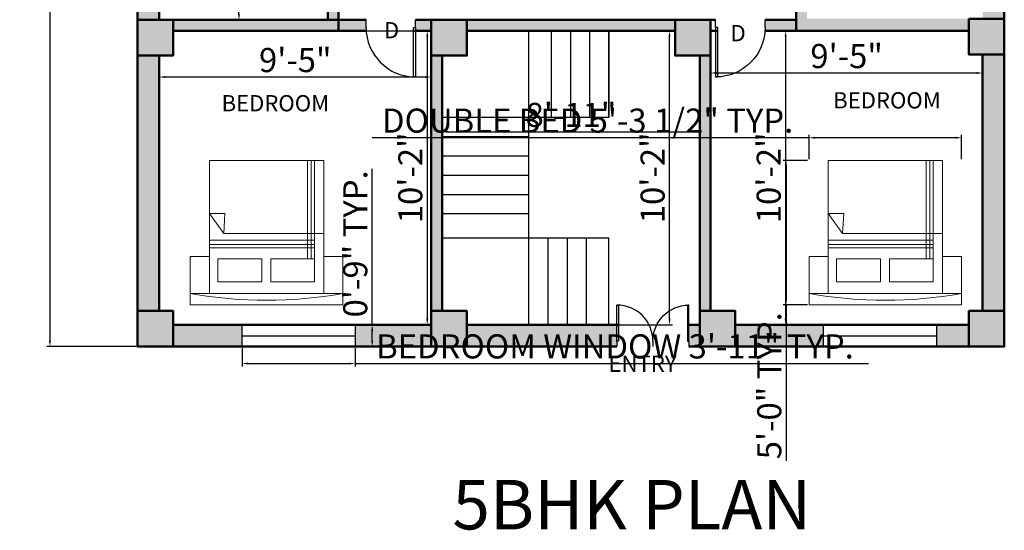
# Model space of a CAD drawing. Units: inches. Extents: x 1864 to 2337, y 2028 to 2650.
# Tile 1 of 2: x 1864 to 2273, y 2028 to 2240. Entities that reach past the tile are written whole.
import ezdxf

# ---------------------------------------------------------------- set-up
doc = ezdxf.new("R2010")
doc.units = ezdxf.units.IN
for name, color, linetype, lineweight in [('A-ANNO-TEXT', 7, 'Continuous', 25), ('A-AREA-IDEN', 7, 'Continuous', 25), ('A-COLS-PATT', 10, 'Continuous', 13), ('A-FLOR-CASE', 7, 'Continuous', 25), ('A-FLOR-STRS', 7, 'Continuous', 25), ('A-WALL-PATT', 144, 'Continuous', 13), ('BED', 220, 'Continuous', 18), ('COLUMN', 10, 'Continuous', 50), ('DIM', 130, 'Continuous', 18), ('WALL', 7, 'Continuous', 50)]:
    doc.layers.add(name, color=color, linetype=linetype, lineweight=lineweight)
doc.layers.add('DOOR', color=50, linetype='Continuous', lineweight=25, plot=False)
doc.layers.add('WINDOW', color=244, linetype='Continuous', lineweight=25, plot=False)
doc.styles.get("Standard").update_dxf_attribs({"font": 'arial.ttf'})
doc.dimstyles.new('ISO-25', dxfattribs={"dimtxt": 10, "dimasz": 2.5, "dimexe": 1.25, "dimexo": 0.625, "dimtad": 1, "dimdec": 0, "dimlunit": 4, "dimtxsty": 'Standard', "dimcen": 2.5, "dimadec": 0, "dimazin": 0, "dimtfac": 1, "dimtdec": 0, "dimtmove": 0, "dimatfit": 3, "dimfxl": 1, "dimarcsym": 0})

# ---------------------------------------------------------------- blocks, each defined once
blk = doc.blocks.new('*U2')
for p, q in [((0, 0), (0, -6)), ((40, 0), (40, -6))]:
    blk.add_line(p, q)
blk.add_lwpolyline([(0, 0), (0, 40), (1.75, 40), (1.75, 0)], close=True)
blk.add_arc((0, 0), 40, 0, 90)
blk = doc.blocks.new('*D18')
at = {"layer": 'Defpoints', "color": 0, "transparency": 16777216}
for p in [(1921.75, 2366.62), (1954.84, 2366.62), (1921.75, 2239.62)]:
    blk.add_point(p, dxfattribs=at)
at = {"layer": 'DIM', "color": 0, "lineweight": -2, "transparency": 16777216}
for p, q in [((1922.38, 2366.62), (1956.09, 2366.62)), ((1954.84, 2242.12), (1954.84, 2364.12)), ((1922.38, 2239.62), (1956.09, 2239.62))]:
    blk.add_line(p, q, dxfattribs=at)
at = {"layer": 'DIM', "color": 0, "transparency": 16777216}
for points in [[(1954.42, 2364.12), (1955.25, 2364.12), (1954.84, 2366.62)], [(1954.42, 2242.12), (1955.25, 2242.12), (1954.84, 2239.62)]]:
    blk.add_solid(points, dxfattribs=at)
at = {"layer": 'DIM', "color": 0, "transparency": 16777216, "insert": (1949.11, 2303.12), "char_height": 10, "attachment_point": 5, "rotation": 90}
blk.add_mtext('10\'-7"', dxfattribs=at)
blk = doc.blocks.new('*D19')
at = {"layer": 'Defpoints', "color": 0, "transparency": 16777216}
for p in [(2034.71, 2215.96), (1921.75, 2118.91), (2034.71, 2118.91)]:
    blk.add_point(p, dxfattribs=at)
at = {"layer": 'DIM', "color": 0, "lineweight": -2, "transparency": 16777216}
for p, q in [((1921.75, 2119.53), (1921.75, 2217.21)), ((2034.71, 2119.53), (2034.71, 2217.21)), ((1924.25, 2215.96), (2032.21, 2215.96))]:
    blk.add_line(p, q, dxfattribs=at)
at = {"layer": 'DIM', "color": 0, "transparency": 16777216}
for points in [[(1924.25, 2216.37), (1924.25, 2215.54), (1921.75, 2215.96)], [(2032.21, 2216.37), (2032.21, 2215.54), (2034.71, 2215.96)]]:
    blk.add_solid(points, dxfattribs=at)
at = {"layer": 'DIM', "color": 0, "transparency": 16777216, "insert": (1978.23, 2221.69), "char_height": 10, "attachment_point": 5}
blk.add_mtext('9\'-5"', dxfattribs=at)
blk = doc.blocks.new('*D20')
at = {"layer": 'Defpoints', "color": 0, "transparency": 16777216}
for p in [(1927.51, 2235.12), (1927.51, 2113.12), (2033.05, 2113.12)]:
    blk.add_point(p, dxfattribs=at)
at = {"layer": 'DIM', "color": 0, "lineweight": -2, "transparency": 16777216}
for p, q in [((1928.14, 2235.12), (2034.3, 2235.12)), ((2033.05, 2232.62), (2033.05, 2115.62)), ((1928.14, 2113.12), (2034.3, 2113.12))]:
    blk.add_line(p, q, dxfattribs=at)
at = {"layer": 'DIM', "color": 0, "transparency": 16777216}
for points in [[(2032.64, 2232.62), (2033.47, 2232.62), (2033.05, 2235.12)], [(2032.64, 2115.62), (2033.47, 2115.62), (2033.05, 2113.12)]]:
    blk.add_solid(points, dxfattribs=at)
at = {"layer": 'DIM', "color": 0, "transparency": 16777216, "insert": (2027.32, 2174.12), "char_height": 10, "attachment_point": 5, "rotation": 90}
blk.add_mtext('10\'-2"', dxfattribs=at)
blk = doc.blocks.new('*D21')
at = {"layer": 'Defpoints', "color": 0, "transparency": 16777216}
for p in [(2049.51, 2235.12), (2133.69, 2235.12), (2049.47, 2113.12)]:
    blk.add_point(p, dxfattribs=at)
at = {"layer": 'DIM', "color": 0, "lineweight": -2, "transparency": 16777216}
for p, q in [((2050.14, 2235.12), (2134.94, 2235.12)), ((2133.69, 2115.62), (2133.69, 2232.62)), ((2050.09, 2113.12), (2134.94, 2113.12))]:
    blk.add_line(p, q, dxfattribs=at)
at = {"layer": 'DIM', "color": 0, "transparency": 16777216}
for points in [[(2133.28, 2232.62), (2134.11, 2232.62), (2133.69, 2235.12)], [(2133.28, 2115.62), (2134.11, 2115.62), (2133.69, 2113.12)]]:
    blk.add_solid(points, dxfattribs=at)
at = {"layer": 'DIM', "color": 0, "transparency": 16777216, "insert": (2127.96, 2174.12), "char_height": 10, "attachment_point": 5, "rotation": 90}
blk.add_mtext('10\'-2"', dxfattribs=at)
blk = doc.blocks.new('*D22')
at = {"layer": 'Defpoints', "color": 0, "transparency": 16777216}
for p in [(2039.25, 2224.83), (2146.25, 2224.83), (2146.25, 2193.19)]:
    blk.add_point(p, dxfattribs=at)
at = {"layer": 'DIM', "color": 0, "lineweight": -2, "transparency": 16777216}
for p, q in [((2039.25, 2224.2), (2039.25, 2191.94)), ((2146.25, 2224.2), (2146.25, 2191.94)), ((2041.75, 2193.19), (2143.75, 2193.19))]:
    blk.add_line(p, q, dxfattribs=at)
at = {"layer": 'DIM', "color": 0, "transparency": 16777216}
for points in [[(2041.75, 2193.61), (2041.75, 2192.78), (2039.25, 2193.19)], [(2143.75, 2193.61), (2143.75, 2192.78), (2146.25, 2193.19)]]:
    blk.add_solid(points, dxfattribs=at)
at = {"layer": 'DIM', "color": 0, "transparency": 16777216, "insert": (2092.75, 2198.93), "char_height": 10, "attachment_point": 5}
blk.add_mtext('8\'-11"', dxfattribs=at)
blk = doc.blocks.new('*D23')
at = {"layer": 'Defpoints', "color": 0, "transparency": 16777216}
for p in [(2263.75, 2217.62), (2150.75, 2118.91), (2263.75, 2118.91)]:
    blk.add_point(p, dxfattribs=at)
at = {"layer": 'DIM', "color": 0, "lineweight": -2, "transparency": 16777216}
for p, q in [((2150.75, 2119.53), (2150.75, 2218.87)), ((2153.25, 2217.62), (2261.25, 2217.62)), ((2263.75, 2119.53), (2263.75, 2218.87))]:
    blk.add_line(p, q, dxfattribs=at)
at = {"layer": 'DIM', "color": 0, "transparency": 16777216}
for points in [[(2153.25, 2218.04), (2153.25, 2217.2), (2150.75, 2217.62)], [(2261.25, 2218.04), (2261.25, 2217.2), (2263.75, 2217.62)]]:
    blk.add_solid(points, dxfattribs=at)
at = {"layer": 'DIM', "color": 0, "transparency": 16777216, "insert": (2207.25, 2223.35), "char_height": 10, "attachment_point": 5}
blk.add_mtext('9\'-5"', dxfattribs=at)
blk = doc.blocks.new('*D24')
at = {"layer": 'Defpoints', "color": 0, "transparency": 16777216}
for p in [(2258, 2235.12), (2181.9, 2113.12), (2258, 2113.12)]:
    blk.add_point(p, dxfattribs=at)
at = {"layer": 'DIM', "color": 0, "lineweight": -2, "transparency": 16777216}
for p, q in [((2257.37, 2235.12), (2180.65, 2235.12)), ((2181.9, 2232.62), (2181.9, 2115.62)), ((2257.37, 2113.12), (2180.65, 2113.12))]:
    blk.add_line(p, q, dxfattribs=at)
at = {"layer": 'DIM', "color": 0, "transparency": 16777216}
for points in [[(2181.48, 2232.62), (2182.32, 2232.62), (2181.9, 2235.12)], [(2181.48, 2115.62), (2182.32, 2115.62), (2181.9, 2113.12)]]:
    blk.add_solid(points, dxfattribs=at)
at = {"layer": 'DIM', "color": 0, "transparency": 16777216, "insert": (2176.17, 2174.12), "char_height": 10, "attachment_point": 5, "rotation": 90}
blk.add_mtext('10\'-2"', dxfattribs=at)
blk = doc.blocks.new('*D26')
at = {"layer": 'Defpoints', "color": 0, "transparency": 16777216}
for p in [(1912.75, 2512.12), (1876.32, 2104.12), (1912.75, 2104.12)]:
    blk.add_point(p, dxfattribs=at)
at = {"layer": 'DIM', "color": 0, "lineweight": -2, "transparency": 16777216}
for p, q in [((1912.13, 2512.12), (1875.07, 2512.12)), ((1876.32, 2509.62), (1876.32, 2106.62)), ((1912.13, 2104.12), (1875.07, 2104.12))]:
    blk.add_line(p, q, dxfattribs=at)
at = {"layer": 'DIM', "color": 0, "transparency": 16777216}
for points in [[(1875.9, 2509.62), (1876.74, 2509.62), (1876.32, 2512.12)], [(1875.9, 2106.62), (1876.74, 2106.62), (1876.32, 2104.12)]]:
    blk.add_solid(points, dxfattribs=at)
at = {"layer": 'DIM', "color": 0, "transparency": 16777216, "insert": (1870.59, 2308.12), "char_height": 10, "attachment_point": 5, "rotation": 90}
blk.add_mtext("34'", dxfattribs=at)
blk = doc.blocks.new('BED-DOUBLE')
for p, q in [((11.74, 40.81), (11.74, 0)), ((13.19, 40.81), (13.19, 0)), ((14.75, 40.81), (14.75, 0)), ((11.74, 36.25), (55.45, 36.25)), ((11.74, 34.82), (55.45, 34.82)), ((11.74, 33.07), (55.45, 33.07)), ((7.92, 30.28), (49.44, 30.28)), ((48.97, 21.97), (49.44, 30.28)), ((49.44, 30.28), (55.45, 21.97)), ((55.45, 21.97), (48.97, 21.97))]:
    blk.add_line(p, q)
for points in [[(0, 55.15), (63.37, 55.15), (63.37, 59.81), (0, 59.81)], [(7.92, 55.15), (0, 55.15), (0, 39.81), (7.92, 39.81)], [(7.92, 55.15), (55.45, 55.15), (55.45, 0), (7.92, 0)], [(63.37, 55.15), (55.45, 55.15), (55.45, 39.81), (63.37, 39.81)], [(11.74, 50.29), (29.99, 50.29), (29.99, 40.81), (11.74, 40.81)], [(33.64, 50.29), (51.9, 50.29), (51.9, 40.81), (33.64, 40.81)]]:
    blk.add_lwpolyline(points, close=True)
blk.add_arc((31.69, -122.73), 180.68, 79.9001, 100.0999)
blk = doc.blocks.new('WIN-BEDROOM')
blk.add_line((0.02, 4.5), (46.93, 4.5))
blk.add_lwpolyline([(0.04, 9), (46.95, 9), (46.91, 0), (0, 0)], close=True)
blk = doc.blocks.new('*D31')
at = {"layer": 'Defpoints', "color": 0, "transparency": 16777216}
for p in [(2191.64, 2190.76), (2191.64, 2181.26), (2255.01, 2181.26)]:
    blk.add_point(p, dxfattribs=at)
at = {"layer": 'DIM', "color": 0, "lineweight": -2, "transparency": 16777216}
for p, q in [((2191.64, 2190.76), (2010.2, 2190.76)), ((2191.64, 2181.88), (2191.64, 2192.01)), ((2252.51, 2190.76), (2194.14, 2190.76)), ((2255.01, 2181.88), (2255.01, 2192.01))]:
    blk.add_line(p, q, dxfattribs=at)
at = {"layer": 'DIM', "color": 0, "transparency": 16777216}
for points in [[(2194.14, 2191.18), (2194.14, 2190.35), (2191.64, 2190.76)], [(2252.51, 2191.18), (2252.51, 2190.35), (2255.01, 2190.76)]]:
    blk.add_solid(points, dxfattribs=at)
at = {"layer": 'DIM', "color": 0, "transparency": 16777216, "insert": (2099.67, 2196.56), "char_height": 10, "attachment_point": 5}
blk.add_mtext('DOUBLE BED 5\'-3 1/2" TYP.', dxfattribs=at)
blk = doc.blocks.new('*D32')
at = {"layer": 'Defpoints', "color": 0, "transparency": 16777216}
for p in [(2191.64, 2181.26), (2182.14, 2121.45), (2191.64, 2121.45)]:
    blk.add_point(p, dxfattribs=at)
at = {"layer": 'DIM', "color": 0, "lineweight": -2, "transparency": 16777216}
for p, q in [((2191.02, 2181.26), (2180.89, 2181.26)), ((2182.14, 2178.76), (2182.14, 2123.95)), ((2191.02, 2121.45), (2180.89, 2121.45)), ((2182.14, 2121.45), (2182.14, 2056.74))]:
    blk.add_line(p, q, dxfattribs=at)
at = {"layer": 'DIM', "color": 0, "transparency": 16777216}
for points in [[(2181.72, 2178.76), (2182.55, 2178.76), (2182.14, 2181.26)], [(2181.72, 2123.95), (2182.55, 2123.95), (2182.14, 2121.45)]]:
    blk.add_solid(points, dxfattribs=at)
at = {"layer": 'DIM', "color": 0, "transparency": 16777216, "insert": (2176.41, 2087.85), "char_height": 10, "attachment_point": 5, "rotation": 90}
blk.add_mtext('5\'-0" TYP.', dxfattribs=at)
blk = doc.blocks.new('*D33')
at = {"layer": 'Defpoints', "color": 0, "transparency": 16777216}
for p in [(1956.19, 2104.12), (2003.14, 2104.12), (2003.14, 2097.07)]:
    blk.add_point(p, dxfattribs=at)
at = {"layer": 'DIM', "color": 0, "lineweight": -2, "transparency": 16777216}
for p, q in [((1956.19, 2103.49), (1956.19, 2095.82)), ((2003.14, 2103.49), (2003.14, 2095.82)), ((1958.69, 2097.07), (2000.64, 2097.07)), ((2003.14, 2097.07), (2216.41, 2097.07))]:
    blk.add_line(p, q, dxfattribs=at)
at = {"layer": 'DIM', "color": 0, "transparency": 16777216}
for points in [[(1958.69, 2097.49), (1958.69, 2096.66), (1956.19, 2097.07)], [(2000.64, 2097.49), (2000.64, 2096.66), (2003.14, 2097.07)]]:
    blk.add_solid(points, dxfattribs=at)
at = {"layer": 'DIM', "color": 0, "transparency": 16777216, "insert": (2111.03, 2102.88), "char_height": 10, "attachment_point": 5}
blk.add_mtext('BEDROOM WINDOW 3\'-11" TYP.', dxfattribs=at)
blk = doc.blocks.new('*D34')
at = {"layer": 'Defpoints', "color": 0, "transparency": 16777216}
for p in [(2003.14, 2113.12), (2010.18, 2113.12), (2003.14, 2104.12)]:
    blk.add_point(p, dxfattribs=at)
at = {"layer": 'DIM', "color": 0, "lineweight": -2, "transparency": 16777216}
for p, q in [((2010.18, 2113.12), (2010.18, 2177.82)), ((2003.77, 2113.12), (2011.43, 2113.12)), ((2010.18, 2106.62), (2010.18, 2110.62)), ((2003.77, 2104.12), (2011.43, 2104.12))]:
    blk.add_line(p, q, dxfattribs=at)
at = {"layer": 'DIM', "color": 0, "transparency": 16777216}
for points in [[(2009.77, 2110.62), (2010.6, 2110.62), (2010.18, 2113.12)], [(2009.77, 2106.62), (2010.6, 2106.62), (2010.18, 2104.12)]]:
    blk.add_solid(points, dxfattribs=at)
at = {"layer": 'DIM', "color": 0, "transparency": 16777216, "insert": (2004.45, 2146.72), "char_height": 10, "attachment_point": 5, "rotation": 90}
blk.add_mtext('0\'-9" TYP.', dxfattribs=at)

msp = doc.modelspace()

# ---------------------------------------------------------------- hatches: boundary and pattern name
at = {"layer": 'A-COLS-PATT'}
h = msp.add_hatch(color=256, dxfattribs=at)
h.dxf.hatch_style = 1
h.paths.add_polyline_path([(1927.51, 2512.12), (1912.75, 2512.12), (1912.75, 2497.33), (1927.51, 2497.33)])
h.paths.add_polyline_path([(2039.25, 2512.12), (2024.5, 2512.12), (2024.5, 2497.35), (2039.25, 2497.35)])
h.paths.add_polyline_path([(2049.51, 2239.62), (2034.75, 2239.62), (2034.75, 2224.83), (2049.51, 2224.83)])
h.paths.add_polyline_path([(2150.75, 2239.62), (2136, 2239.62), (2136, 2224.83), (2150.75, 2224.83)])
h.paths.add_polyline_path([(2272.75, 2240.1), (2258, 2240.1), (2258, 2225.31), (2272.75, 2225.31)])
h.paths.add_polyline_path([(2272.75, 2118.91), (2258, 2118.91), (2258, 2104.12), (2272.75, 2104.12)])
h.paths.add_polyline_path([(2161.01, 2118.91), (2146.25, 2118.91), (2146.25, 2104.12), (2161.01, 2104.12)])
h.paths.add_polyline_path([(2049.47, 2118.91), (2034.75, 2118.91), (2034.75, 2113.12), (2034.71, 2104.12), (2049.47, 2104.12)])
h.paths.add_polyline_path([(1927.51, 2118.91), (1912.75, 2118.91), (1912.75, 2104.12), (1927.51, 2104.12)])
h.paths.add_polyline_path([(1927.51, 2239.62), (1912.75, 2239.62), (1912.75, 2224.83), (1927.51, 2224.83)])
h.paths.add_polyline_path([(1927.51, 2381.41), (1912.75, 2381.41), (1912.75, 2366.62), (1927.51, 2366.62)])
h.paths.add_polyline_path([(2272.75, 2512.12), (2258, 2512.12), (2258, 2497.33), (2272.75, 2497.33)])
h.paths.add_polyline_path([(2170.98, 2512.12), (2156.22, 2512.12), (2156.22, 2503.12), (2156.25, 2503.12), (2156.25, 2497.33), (2170.98, 2497.33)])
at = {"layer": 'A-WALL-PATT'}
h = msp.add_hatch(color=256, dxfattribs=at)
h.dxf.hatch_style = 1
h.paths.add_polyline_path([(1921.75, 2224.83), (1912.75, 2224.83), (1912.75, 2118.91), (1921.75, 2118.91)])
h.paths.add_polyline_path([(2039.25, 2224.83), (2034.75, 2224.83), (2034.75, 2118.91), (2039.25, 2118.91)])
h.paths.add_polyline_path([(2150.75, 2224.83), (2146.25, 2224.83), (2146.25, 2118.91), (2150.75, 2118.91)])
h.paths.add_polyline_path([(2272.75, 2225.31), (2263.75, 2225.31), (2263.75, 2118.91), (2272.75, 2118.91)])
h.paths.add_polyline_path([(2258, 2240.12), (2190.75, 2240.12), (2190.75, 2244.03), (2189.34, 2244.03), (2186.25, 2244.03), (2186.25, 2235.62), (2186.25, 2235.12), (2228.41, 2235.12), (2258, 2235.12)])
h.paths.add_polyline_path([(2190.75, 2301.12), (2186.25, 2301.12), (2186.25, 2264.6), (2189.34, 2264.6, -0.017198), (2190.75, 2264.55)])
h.paths.add_polyline_path([(2136, 2239.62), (2049.51, 2239.62), (2049.51, 2235.12), (2136, 2235.12)])
h.paths.add_polyline_path([(2186.25, 2239.62), (2173.41, 2239.62), (2173.41, 2236.53, -0.017198), (2173.36, 2235.12), (2186.25, 2235.12), (2186.25, 2235.62)])
h.paths.add_polyline_path([(1996.25, 2239.62), (1991.75, 2239.62), (1927.51, 2239.62), (1927.51, 2235.12), (1996.25, 2235.12)])
h.paths.add_polyline_path([(2007.65, 2239.62), (1996.25, 2239.62), (1996.25, 2235.12), (2007.7, 2235.12, -0.017198), (2007.65, 2236.53)])
h.paths.add_polyline_path([(2010.85, 2369.7, -0.017198), (2010.89, 2371.12), (1927.51, 2371.12), (1927.51, 2366.62), (2010.85, 2366.62)])
h.paths.add_polyline_path([(1996.25, 2366.62), (1991.75, 2366.62), (1991.75, 2338.77), (1996.25, 2338.77)])
h.paths.add_polyline_path([(2121.41, 2369.7, -0.017198), (2121.46, 2371.12), (2047.12, 2371.12), (2047.12, 2366.62), (2121.41, 2366.62)])
h.paths.add_polyline_path([(2258, 2371.12), (2184.04, 2371.12, -0.017198), (2184.09, 2369.7), (2184.09, 2366.62), (2258, 2366.62)])
h.paths.add_polyline_path([(2190.75, 2366.62), (2186.25, 2366.62), (2186.25, 2360.91), (2189.34, 2360.91), (2190.75, 2360.91)])
h.paths.add_polyline_path([(2190.75, 2340.39, -0.017198), (2189.34, 2340.34), (2186.25, 2340.34), (2186.25, 2301.12), (2190.75, 2301.12), (2263.75, 2301.12), (2263.75, 2305.62), (2190.75, 2305.62)])
h.paths.add_polyline_path([(2272.75, 2497.33), (2263.75, 2497.33), (2263.75, 2381.41), (2272.75, 2381.41)])
h.paths.add_polyline_path([(2160.75, 2497.33), (2156.25, 2497.33), (2156.25, 2381.41), (2160.75, 2381.41)])
h.paths.add_polyline_path([(2039.25, 2497.35), (2034.75, 2497.35), (2034.75, 2381.41), (2039.25, 2381.41)])
h.paths.add_polyline_path([(1921.75, 2497.33), (1912.75, 2497.33), (1912.75, 2381.41), (1921.75, 2381.41)])
h.paths.add_polyline_path([(2111.85, 2104.12), (2111.85, 2106.36), (2112.5, 2106.36), (2112.5, 2113.12), (2049.47, 2113.12), (2049.47, 2104.12)])
h.paths.add_polyline_path([(2141.1, 2113.12), (2141.1, 2106.36), (2141.75, 2106.36), (2141.75, 2104.12), (2146.25, 2104.12), (2146.25, 2113.12)])
h.paths.add_polyline_path([(1996.08, 2512.12), (1996.04, 2503.12), (2024.5, 2503.12), (2024.5, 2512.12)])
h.paths.add_polyline_path([(1949.13, 2503.12), (1949.17, 2512.12), (1927.51, 2512.12), (1927.51, 2503.12)])
h.paths.add_polyline_path([(2122.88, 2512.12), (2122.84, 2503.12), (2156.22, 2503.12), (2156.22, 2512.12)])
h.paths.add_polyline_path([(2075.93, 2503.12), (2075.97, 2512.12), (2039.25, 2512.12), (2039.25, 2503.12)])
h.paths.add_polyline_path([(2245.62, 2512.12), (2245.58, 2503.12), (2258, 2503.12), (2258, 2512.12)])
h.paths.add_polyline_path([(2198.67, 2503.12), (2198.71, 2512.12), (2170.98, 2512.12), (2170.98, 2503.12)])
h.paths.add_polyline_path([(2263.75, 2352.2), (2272.75, 2352.2), (2272.75, 2366.62), (2263.75, 2366.62)])
h.paths.add_polyline_path([(2272.75, 2252.38), (2263.75, 2252.38), (2263.75, 2240.1), (2272.75, 2240.1)])
h.paths.add_polyline_path([(2263.75, 2289.97), (2272.75, 2289.97), (2272.75, 2314.61), (2263.75, 2314.61)])
h.paths.add_polyline_path([(2197.66, 2104.12), (2197.7, 2113.12), (2161.01, 2113.12), (2161.01, 2104.12)])
h.paths.add_polyline_path([(2244.61, 2113.12), (2244.57, 2104.12), (2258, 2104.12), (2258, 2113.12)])
h.paths.add_polyline_path([(1956.19, 2104.12), (1956.23, 2113.12), (1927.51, 2113.12), (1927.51, 2104.12)])
h.paths.add_polyline_path([(2003.14, 2113.12), (2003.1, 2104.12), (2034.71, 2104.12), (2034.71, 2113.12)])
h.paths.add_polyline_path([(1921.75, 2289.34), (1912.75, 2289.34), (1912.75, 2239.62), (1921.75, 2239.62)])
h.paths.add_polyline_path([(1912.75, 2326.93), (1921.75, 2326.93), (1921.75, 2366.62), (1912.75, 2366.62)])
h = msp.add_hatch(color=256, dxfattribs=at)
h.dxf.hatch_style = 1
h.paths.add_polyline_path([(2034.75, 2239.62), (2028.22, 2239.62), (2028.22, 2236.53), (2028.22, 2235.12), (2034.75, 2235.12)])
h.paths.add_polyline_path([(1996.25, 2268.5), (1991.75, 2268.5), (1991.75, 2239.62), (1996.25, 2239.62)])

# ---------------------------------------------------------------- linework, layer by layer
at = {"layer": 'A-FLOR-CASE'}
msp.add_line((1991.75, 2239.62), (1991.75, 2263.62), dxfattribs=at)
at = {"layer": 'A-FLOR-STRS'}
for p, q in [((2075.25, 2199.12), (2075.25, 2235.12)), ((2084.51, 2235.12), (2084.51, 2199.12)), ((2092.51, 2235.12), (2092.51, 2199.12)), ((2100.51, 2235.12), (2100.51, 2199.12)), ((2108.51, 2235.12), (2108.51, 2199.12)), ((2108.51, 2199.12), (2108.51, 2235.12)), ((2075.25, 2199.12), (2039.25, 2199.12)), ((2108.51, 2199.12), (2075.25, 2199.12)), ((2075.25, 2113.12), (2075.25, 2199.12)), ((2075.25, 2191.12), (2039.25, 2191.12)), ((2075.25, 2183.12), (2039.25, 2183.12)), ((2075.25, 2175.12), (2039.25, 2175.12)), ((2075.25, 2167.12), (2039.25, 2167.12)), ((2075.25, 2159.12), (2039.25, 2159.12)), ((2075.25, 2149.12), (2039.25, 2149.12)), ((2108.51, 2149.12), (2075.25, 2149.12)), ((2083.25, 2113.12), (2083.25, 2149.12)), ((2091.25, 2113.12), (2091.25, 2149.12)), ((2099.25, 2113.12), (2099.25, 2149.12)), ((2108.51, 2113.12), (2108.51, 2149.12)), ((2108.51, 2113.12), (2108.51, 2149.12)), ((2049.47, 2113.12), (2075.25, 2113.12))]:
    msp.add_line(p, q, dxfattribs=at)
at = {"layer": 'COLUMN'}
for points in [[(1912.75, 2239.62), (1927.51, 2239.62), (1927.51, 2224.83), (1912.75, 2224.83)], [(2034.75, 2239.62), (2049.51, 2239.62), (2049.51, 2224.83), (2034.75, 2224.83)], [(2136, 2239.62), (2150.75, 2239.62), (2150.75, 2224.83), (2136, 2224.83)], [(2258, 2240.1), (2272.75, 2240.1), (2272.75, 2225.31), (2258, 2225.31)], [(1912.75, 2118.91), (1927.51, 2118.91), (1927.51, 2104.12), (1912.75, 2104.12)], [(2034.71, 2118.91), (2049.47, 2118.91), (2049.47, 2104.12), (2034.71, 2104.12)], [(2146.25, 2118.91), (2161.01, 2118.91), (2161.01, 2104.12), (2146.25, 2104.12)], [(2258, 2118.91), (2272.75, 2118.91), (2272.75, 2104.12), (2258, 2104.12)]]:
    msp.add_lwpolyline(points, close=True, dxfattribs=at)
at = {"layer": 'WALL'}
for p, q in [((1991.75, 2268.5), (1991.75, 2239.62)), ((1996.25, 2268.5), (1996.25, 2235.12)), ((2186.25, 2235.62), (2186.25, 2244.03)), ((1991.75, 2239.62), (1921.75, 2239.62)), ((1991.75, 2239.62), (1996.25, 2239.62)), ((2034.75, 2235.12), (2034.75, 2239.62)), ((2034.75, 2239.62), (2150.75, 2239.62)), ((2150.75, 2235.12), (2150.75, 2239.62)), ((2150.75, 2239.62), (2152.84, 2239.62)), ((2173.41, 2239.62), (2186.25, 2239.62)), ((1996.25, 2235.12), (1927.51, 2235.12)), ((2034.75, 2113.12), (2034.75, 2235.12)), ((2049.51, 2235.12), (2136, 2235.12)), ((2150.75, 2118.91), (2150.75, 2235.12)), ((2150.75, 2235.12), (2153.74, 2235.12)), ((2173.36, 2235.12), (2228.41, 2235.12)), ((2186.25, 2235.62), (2186.25, 2235.12)), ((2186.25, 2235.12), (2258, 2235.12)), ((2039.25, 2118.91), (2039.25, 2224.83)), ((2146.25, 2113.12), (2146.25, 2224.83)), ((1927.51, 2113.12), (2034.75, 2113.12)), ((2258, 2113.12), (2161.01, 2113.12))]:
    msp.add_line(p, q, dxfattribs=at)
for points in [[(2141.75, 2104.12), (2272.75, 2104.12), (2272.75, 2512.12), (1912.75, 2512.12), (1912.75, 2104.12), (2111.85, 2104.12)], [(1921.75, 2366.62), (1921.75, 2239.62)], [(2007.65, 2239.62), (1996.25, 2239.62), (1996.25, 2235.12), (2007.7, 2235.12)], [(2027.32, 2235.12), (2034.75, 2235.12), (2034.75, 2239.62), (2028.22, 2239.62)], [(2263.75, 2118.91), (2263.75, 2225.31)], [(1921.75, 2224.83), (1921.75, 2118.91)], [(1927.51, 2113.12), (2034.75, 2113.12)], [(2049.47, 2113.12), (2112.5, 2113.12)], [(2141.1, 2113.12), (2146.25, 2113.12)], [(2161.01, 2113.12), (2258, 2113.12)]]:
    msp.add_lwpolyline(points, dxfattribs=at)

# ---------------------------------------------------------------- block references
at = {"layer": 'BED', "rotation": 180}
for p in [(1998.02, 2181.26), (2255.01, 2181.26)]:
    msp.add_blockref('BED-DOUBLE', p, dxfattribs=at)
at = {"layer": 'DOOR', "yscale": 0.514332689134197, "zscale": 0.514332689134197, "rotation": 180}
for p, xscale in [((2028.22, 2236.53), 0.514332689134197), ((2152.84, 2236.53), -0.514332689134197)]:
    msp.add_blockref('*U2', p, dxfattribs=dict(at, xscale=xscale))
at = {"layer": 'DOOR', "yscale": 0.3737851321308048, "zscale": 0.3737851321308048}
for p, xscale in [((2111.85, 2106.36), 0.3737851321308048), ((2141.75, 2106.36), -0.3737851321308048)]:
    msp.add_blockref('*U2', p, dxfattribs=dict(at, xscale=xscale))
at = {"layer": 'WINDOW'}
for p in [(1956.19, 2104.12), (2197.66, 2104.12)]:
    msp.add_blockref('WIN-BEDROOM', p, dxfattribs=at)

# ---------------------------------------------------------------- texts
at = {"layer": 'A-ANNO-TEXT', "attachment_point": 1}
for s, width, gutter_width, insert, char_height in [('D', 141.616, 33.65, (2015.09, 2238.73), 6.73), ('D', 141.616, 33.65, (2159.03, 2237.51), 6.73), ('5BHK PLAN', 1827.29, 102.71, (2043.53, 2048.79), 20.542)]:
    msp.add_mtext_dynamic_manual_height_columns(s, width=width, gutter_width=gutter_width, heights=[0], dxfattribs=dict(at, insert=insert, char_height=char_height))
at = {"layer": 'A-AREA-IDEN', "char_height": 6.73, "attachment_point": 1}
for s, insert in [('BEDROOM', (1947.63, 2208.44)), ('BEDROOM', (2201.68, 2209.64)), ('ENTRY', (2108.37, 2100.33))]:
    msp.add_mtext_dynamic_manual_height_columns(s, width=141.616, gutter_width=33.65, heights=[0], dxfattribs=dict(at, insert=insert))

# ---------------------------------------------------------------- dimensions: what is measured, and where the dimension line sits
at = {"layer": 'DIM'}
for base, p1, p2, picture, middle in [((1876.32, 2104.12), (1912.75, 2512.12), (1912.75, 2104.12), '*D26', (1870.59, 2308.12)), ((1954.84, 2366.62), (1921.75, 2239.62), (1921.75, 2366.62), '*D18', (1949.11, 2303.12)), ((2033.05, 2113.12), (1927.51, 2235.12), (1927.51, 2113.12), '*D20', (2027.32, 2174.12)), ((2133.69, 2235.12), (2049.47, 2113.12), (2049.51, 2235.12), '*D21', (2127.96, 2174.12)), ((2181.9, 2113.12), (2258, 2235.12), (2258, 2113.12), '*D24', (2176.17, 2174.12))]:
    dim = msp.add_linear_dim(base=base, p1=p1, p2=p2, angle=90, dimstyle='ISO-25', override={"dimclrd": 0, "dimclre": 0, "dimclrt": 0}, dxfattribs=at)
    dim.commit()
    dim.dimension.update_dxf_attribs({"geometry": picture, "text_midpoint": middle})
for base, p1, p2, angle, text, picture, middle in [((2191.64, 2190.76), (2255.01, 2181.26), (2191.64, 2181.26), 180, 'DOUBLE BED <> TYP.', '*D31', (2099.67, 2196.56)), ((2182.14, 2121.45), (2191.64, 2181.26), (2191.64, 2121.45), 270, '<> TYP.', '*D32', (2176.41, 2087.85)), ((2010.18, 2113.12), (2003.14, 2104.12), (2003.14, 2113.12), 90, '<> TYP.', '*D34', (2004.45, 2146.72))]:
    dim = msp.add_linear_dim(base=base, p1=p1, p2=p2, angle=angle, text=text, dimstyle='ISO-25', override={"dimdec": 1, "dimlfac": 1, "dimrnd": 0, "dimzin": 1, "dimdsep": 46, "dimlunit": 4, "dimfrac": 2}, dxfattribs=at)
    dim.commit()
    dim.dimension.update_dxf_attribs({"geometry": picture, "text_midpoint": middle})
for base, p1, p2, picture, middle in [((2263.75, 2217.62), (2150.75, 2118.91), (2263.75, 2118.91), '*D23', (2207.25, 2223.35)), ((2034.71, 2215.96), (1921.75, 2118.91), (2034.71, 2118.91), '*D19', (1978.23, 2221.69)), ((2146.25, 2193.19), (2039.25, 2224.83), (2146.25, 2224.83), '*D22', (2092.75, 2198.93))]:
    dim = msp.add_linear_dim(base=base, p1=p1, p2=p2, dimstyle='ISO-25', override={"dimclrd": 0, "dimclre": 0, "dimclrt": 0}, dxfattribs=at)
    dim.commit()
    dim.dimension.update_dxf_attribs({"geometry": picture, "text_midpoint": middle})
dim = msp.add_linear_dim(base=(2003.1403, 2097.0741), p1=(1956.1906, 2104.1166), p2=(2003.1403, 2104.1166), text='BEDROOM WINDOW <> TYP.', dimstyle='ISO-25', override={"dimdec": 1, "dimlfac": 1, "dimrnd": 0, "dimzin": 1, "dimdsep": 46, "dimlunit": 4, "dimfrac": 2}, dxfattribs=at)
dim.commit()
dim.dimension.update_dxf_attribs({"geometry": '*D33', "text_midpoint": (2111.0266, 2102.8765)})

doc.saveas('drawing.dxf')
